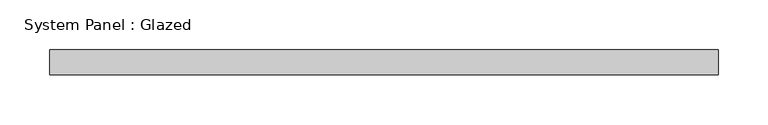
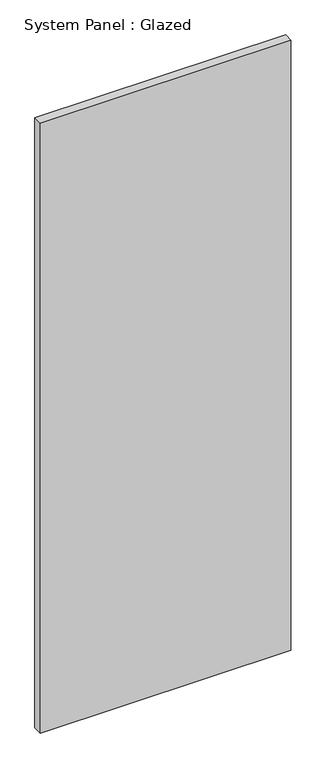
"""IFC4 building model written with IfcOpenShell, lengths in millimetres: plate geometry, System Panel : Glazed."""

from ifc_helpers import new_model, si_unit, origin, origin_with_axes, place, context, project, spatial, polyline, outline, extrude, source, transform, mapped, element, save


def system_panel_glazed_70269732(model_context):
    return source(origin(), model_context, "Body", "SweptSolid", [
        extrude(outline(polyline([(337.2685902, 19.05), (-337.2685902, 19.05), (-337.2685902, 44.45), (337.2685902, 44.45), (337.2685902, 19.05)])), origin_with_axes(), (0.0, 0.0, 1.0), 1735.2548712),
    ])


if __name__ == "__main__":
    model = new_model("IFC4")
    model_context = context("Model", 3, world=origin())
    ifc_project = project(units=[si_unit("LENGTHUNIT", "METRE", prefix="MILLI")], contexts=[model_context])
    site = spatial("IfcSite", under=ifc_project)
    building = spatial("IfcBuilding", under=site)
    placement = place(None, origin())
    system_panel_glazed_shape = system_panel_glazed_70269732(model_context)
    element("IfcPlate", 1, ObjectType="System Panel : Glazed", at=placement, inside=building, context=model_context, shape_type="MappedRepresentation", body=[
        mapped(system_panel_glazed_shape, transform((0.0, 0.0, 0.0), x_axis=(1.0, 0.0, 0.0), y_axis=(0.0, 1.0, 0.0), z_axis=(0.0, 0.0, 1.0))),
    ])
    save(model, "model.ifc")

# Revit data of these elements
# Type "System Panel : Glazed"
#   Construction Type Id = "GSP4R"
#   Analytic Construction = "1/8 in Pilkington single glazing"
#   Visual Light Transmittance = 0.9
#   Solar Heat Gain Coefficient = 0.86
#   Heat Transfer Coefficient (U) = 1.18115 BTU/(h·ft²·°F)
#   Define Thermal Properties by = 1
# Element 1 (IfcPlate, "System Panel : Glazed")
#   Materials on its faces: "Glass"
# Materials
#   "Glass": class "Glass", colour RGB 0 128 192, transparency 0.75, Description = "Soda Lime Glass", Cost = 0
